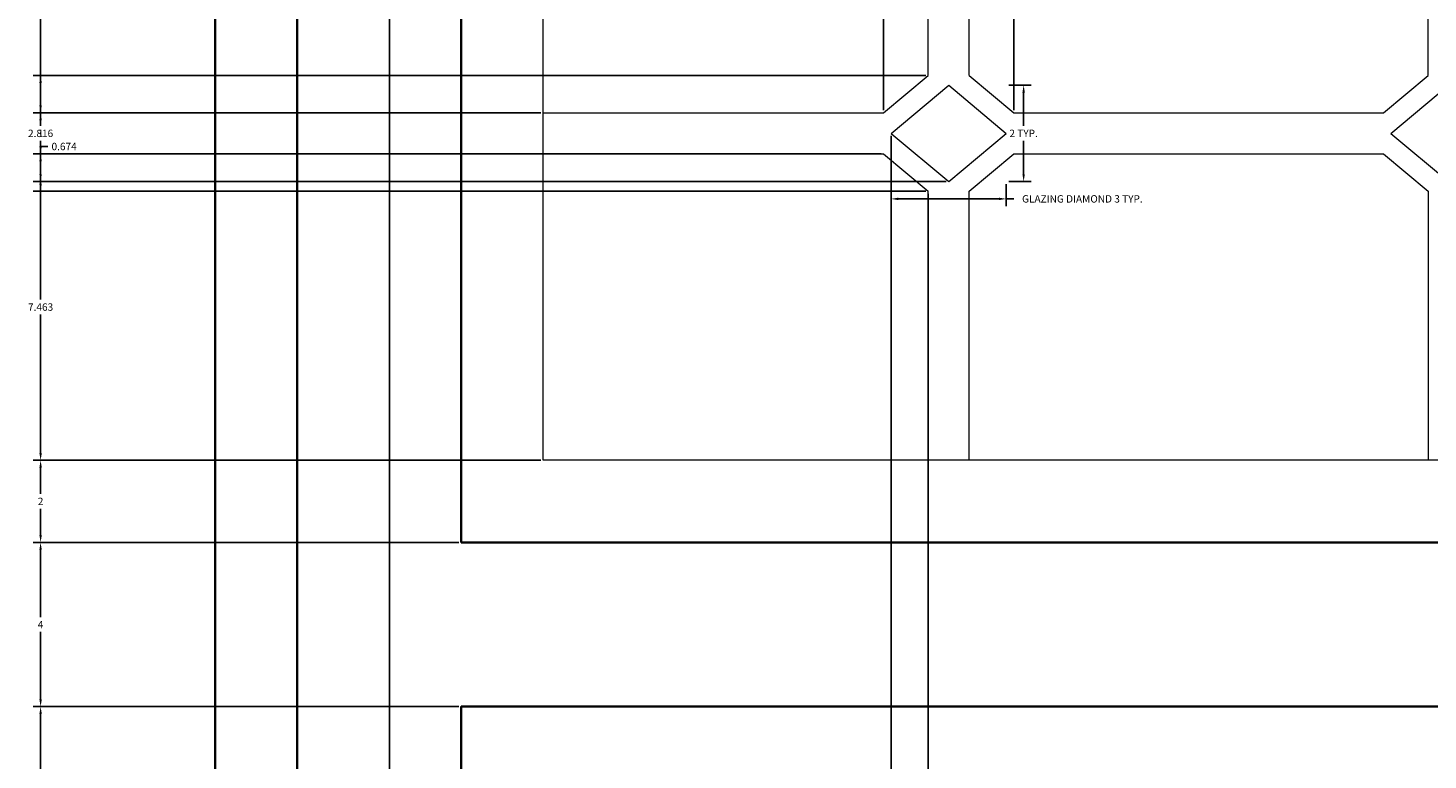
# Model space of a CAD drawing. Units: inches. Extents: x 3137 to 3299, y 1994 to 2089.
# Tile 5 of 14: x 3137 to 3171, y 2052 to 2069. Entities that reach past the tile are written whole.
import ezdxf

# ---------------------------------------------------------------- set-up
doc = ezdxf.new("R2010")
doc.units = ezdxf.units.IN
doc.header["$MEASUREMENT"] = 0
for name, color, linetype, lineweight in [('A-ANNO-DIMS', 2, 'Continuous', 18), ('A-DOOR', 4, 'Continuous', 35), ('A-GLAZ', 3, 'Continuous', 18)]:
    doc.layers.add(name, color=color, linetype=linetype, lineweight=lineweight)
doc.styles.get("Standard").update_dxf_attribs({"font": 'arial.ttf'})
doc.dimstyles.get("Standard").update_dxf_attribs({"dimtxt": 0.18, "dimasz": 0.18, "dimexe": 0.18, "dimexo": 0.0625, "dimgap": 0.09, "dimtad": 0, "dimtih": 1, "dimtoh": 1, "dimdec": 4, "dimzin": 0, "dimdsep": 46, "dimtxsty": 'Standard', "dimcen": 0.09, "dimadec": 0, "dimazin": 0, "dimtfac": 1, "dimtdec": 4, "dimtofl": 0, "dimtmove": 0, "dimatfit": 3, "dimfxl": 1, "dimtolj": 1, "dimtzin": 0, "dimarcsym": 0})

# ---------------------------------------------------------------- blocks, each defined once
blk = doc.blocks.new('GLAZ-DIAMOND-MOTIF')
for points in [[(0, 1.174), (1.407, 2.349)], [(1.407, 2.349), (2.809, 1.174)], [(0, 1.174), (1.407, 0)], [(1.407, 0), (2.809, 1.174)]]:
    blk.add_lwpolyline(points)
blk = doc.blocks.new('*D11')
at = {"layer": 'A-ANNO-DIMS', "color": 0, "lineweight": -2, "transparency": 16777216}
for p, q in [((3157.951, 2065.674), (3157.951, 2065.135)), ((3160.76, 2065.674), (3160.76, 2065.135)), ((3158.131, 2065.315), (3160.58, 2065.315)), ((3160.76, 2065.315), (3160.94, 2065.315))]:
    blk.add_line(p, q, dxfattribs=at)
at = {"layer": 'A-ANNO-DIMS', "color": 0, "transparency": 16777216}
for points in [[(3158.131, 2065.345), (3158.131, 2065.285), (3157.951, 2065.315)], [(3160.58, 2065.345), (3160.58, 2065.285), (3160.76, 2065.315)]]:
    blk.add_solid(points, dxfattribs=at)
at = {"layer": 'Defpoints', "color": 0, "transparency": 16777216}
for p in [(3157.951, 2065.737), (3160.76, 2065.737), (3160.76, 2065.315)]:
    blk.add_point(p, dxfattribs=at)
at = {"layer": 'A-ANNO-DIMS', "color": 0, "transparency": 16777216, "insert": (3162.613, 2065.315), "char_height": 0.18, "attachment_point": 5}
blk.add_mtext('\\A1;GLAZING DIAMOND 3 TYP.', dxfattribs=at)
blk = doc.blocks.new('*D12')
at = {"layer": 'A-ANNO-DIMS', "color": 0, "lineweight": -2, "transparency": 16777216}
for p, q in [((3160.823, 2068.086), (3161.362, 2068.086)), ((3161.182, 2067.906), (3161.182, 2067.092)), ((3161.182, 2065.917), (3161.182, 2066.731)), ((3160.823, 2065.737), (3161.362, 2065.737))]:
    blk.add_line(p, q, dxfattribs=at)
at = {"layer": 'A-ANNO-DIMS', "color": 0, "transparency": 16777216}
for points in [[(3161.152, 2067.906), (3161.212, 2067.906), (3161.182, 2068.086)], [(3161.152, 2065.917), (3161.212, 2065.917), (3161.182, 2065.737)]]:
    blk.add_solid(points, dxfattribs=at)
at = {"layer": 'Defpoints', "color": 0, "transparency": 16777216}
for p in [(3160.76, 2068.086), (3161.182, 2068.086), (3160.76, 2065.737)]:
    blk.add_point(p, dxfattribs=at)
at = {"layer": 'A-ANNO-DIMS', "color": 0, "transparency": 16777216, "insert": (3161.182, 2066.911), "char_height": 0.18, "attachment_point": 5}
blk.add_mtext('\\A1;2 TYP.', dxfattribs=at)
blk = doc.blocks.new('*D42')
at = {"layer": 'A-ANNO-DIMS', "color": 0, "lineweight": -2, "transparency": 16777216}
for p, q in [((3147.415, 2052.948), (3137.048, 2052.948)), ((3137.228, 2052.768), (3137.228, 2042.725)), ((3137.228, 2032.318), (3137.228, 2042.361)), ((3147.415, 2032.138), (3137.048, 2032.138))]:
    blk.add_line(p, q, dxfattribs=at)
at = {"layer": 'A-ANNO-DIMS', "color": 0, "transparency": 16777216}
for points in [[(3137.198, 2052.768), (3137.258, 2052.768), (3137.228, 2052.948)], [(3137.198, 2032.318), (3137.258, 2032.318), (3137.228, 2032.138)]]:
    blk.add_solid(points, dxfattribs=at)
at = {"layer": 'Defpoints', "color": 0, "transparency": 16777216}
for p in [(3137.228, 2052.948), (3147.478, 2052.948), (3147.478, 2032.138)]:
    blk.add_point(p, dxfattribs=at)
at = {"layer": 'A-ANNO-DIMS', "color": 0, "transparency": 16777216, "insert": (3137.228, 2042.543), "char_height": 0.18, "attachment_point": 5}
blk.add_mtext('\\A1;20.81', dxfattribs=at)
blk = doc.blocks.new('*D43')
at = {"layer": 'A-ANNO-DIMS', "color": 0, "lineweight": -2, "transparency": 16777216}
for p, q in [((3147.415181, 2056.948298), (3137.047681, 2056.948298)), ((3137.227681, 2056.768298), (3137.227681, 2055.128298)), ((3137.227681, 2053.128298), (3137.227681, 2054.768298)), ((3147.415181, 2052.948298), (3137.047681, 2052.948298))]:
    blk.add_line(p, q, dxfattribs=at)
at = {"layer": 'A-ANNO-DIMS', "color": 0, "transparency": 16777216}
for points in [[(3137.197681, 2056.768298), (3137.257681, 2056.768298), (3137.227681, 2056.948298)], [(3137.197681, 2053.128298), (3137.257681, 2053.128298), (3137.227681, 2052.948298)]]:
    blk.add_solid(points, dxfattribs=at)
at = {"layer": 'Defpoints', "color": 0, "transparency": 16777216}
for p in [(3137.227681, 2056.948298), (3147.477681, 2056.948298), (3147.477681, 2052.948298)]:
    blk.add_point(p, dxfattribs=at)
at = {"layer": 'A-ANNO-DIMS', "color": 0, "transparency": 16777216, "insert": (3137.227681, 2054.948298), "char_height": 0.18, "attachment_point": 5}
blk.add_mtext('\\A1;4', dxfattribs=at)
blk = doc.blocks.new('*D44')
at = {"layer": 'A-ANNO-DIMS', "color": 0, "lineweight": -2, "transparency": 16777216}
for p, q in [((3149.415, 2058.948), (3137.048, 2058.948)), ((3137.228, 2058.768), (3137.228, 2058.129)), ((3137.228, 2057.128), (3137.228, 2057.768)), ((3147.415, 2056.948), (3137.048, 2056.948))]:
    blk.add_line(p, q, dxfattribs=at)
at = {"layer": 'A-ANNO-DIMS', "color": 0, "transparency": 16777216}
for points in [[(3137.198, 2058.768), (3137.258, 2058.768), (3137.228, 2058.948)], [(3137.198, 2057.128), (3137.258, 2057.128), (3137.228, 2056.948)]]:
    blk.add_solid(points, dxfattribs=at)
at = {"layer": 'Defpoints', "color": 0, "transparency": 16777216}
for p in [(3137.228, 2058.948), (3149.478, 2058.948), (3147.478, 2056.948)]:
    blk.add_point(p, dxfattribs=at)
at = {"layer": 'A-ANNO-DIMS', "color": 0, "transparency": 16777216, "insert": (3137.228, 2057.948), "char_height": 0.18, "attachment_point": 5}
blk.add_mtext('\\A1;2', dxfattribs=at)
blk = doc.blocks.new('*D45')
at = {"layer": 'A-ANNO-DIMS', "color": 0, "lineweight": -2, "transparency": 16777216}
for p, q in [((3149.415, 2066.411), (3137.048, 2066.411)), ((3137.228, 2066.231), (3137.228, 2062.862)), ((3137.228, 2059.128), (3137.228, 2062.498)), ((3149.415, 2058.948), (3137.048, 2058.948))]:
    blk.add_line(p, q, dxfattribs=at)
at = {"layer": 'A-ANNO-DIMS', "color": 0, "transparency": 16777216}
for points in [[(3137.198, 2066.231), (3137.258, 2066.231), (3137.228, 2066.411)], [(3137.198, 2059.128), (3137.258, 2059.128), (3137.228, 2058.948)]]:
    blk.add_solid(points, dxfattribs=at)
at = {"layer": 'Defpoints', "color": 0, "transparency": 16777216}
for p in [(3137.228, 2066.411), (3149.478, 2066.411), (3149.478, 2058.948)]:
    blk.add_point(p, dxfattribs=at)
at = {"layer": 'A-ANNO-DIMS', "color": 0, "transparency": 16777216, "insert": (3137.228, 2062.68), "char_height": 0.18, "attachment_point": 5}
blk.add_mtext('\\A1;7.463', dxfattribs=at)
blk = doc.blocks.new('*D46')
at = {"layer": 'A-ANNO-DIMS', "color": 0, "lineweight": -2, "transparency": 16777216}
for p, q in [((3149.415, 2067.411), (3137.048, 2067.411)), ((3137.228, 2067.231), (3137.228, 2067.092)), ((3137.228, 2066.591), (3137.228, 2066.731)), ((3149.415, 2066.411), (3137.048, 2066.411))]:
    blk.add_line(p, q, dxfattribs=at)
at = {"layer": 'A-ANNO-DIMS', "color": 0, "transparency": 16777216}
for points in [[(3137.198, 2067.231), (3137.258, 2067.231), (3137.228, 2067.411)], [(3137.198, 2066.591), (3137.258, 2066.591), (3137.228, 2066.411)]]:
    blk.add_solid(points, dxfattribs=at)
at = {"layer": 'Defpoints', "color": 0, "transparency": 16777216}
for p in [(3137.228, 2067.411), (3149.478, 2067.411), (3149.478, 2066.411)]:
    blk.add_point(p, dxfattribs=at)
at = {"layer": 'A-ANNO-DIMS', "color": 0, "transparency": 16777216, "insert": (3137.228, 2066.911), "char_height": 0.18, "attachment_point": 5}
blk.add_mtext('\\A1;1', dxfattribs=at)
blk = doc.blocks.new('*D47')
at = {"layer": 'A-ANNO-DIMS', "color": 0, "lineweight": -2, "transparency": 16777216}
for p, q in [((3149.415, 2074.874), (3137.048, 2074.874)), ((3137.228, 2074.694), (3137.228, 2071.325)), ((3137.228, 2067.591), (3137.228, 2070.961)), ((3149.415, 2067.411), (3137.048, 2067.411))]:
    blk.add_line(p, q, dxfattribs=at)
at = {"layer": 'A-ANNO-DIMS', "color": 0, "transparency": 16777216}
for points in [[(3137.198, 2074.694), (3137.258, 2074.694), (3137.228, 2074.874)], [(3137.198, 2067.591), (3137.258, 2067.591), (3137.228, 2067.411)]]:
    blk.add_solid(points, dxfattribs=at)
at = {"layer": 'Defpoints', "color": 0, "transparency": 16777216}
for p in [(3137.228, 2074.874), (3149.478, 2074.874), (3149.478, 2067.411)]:
    blk.add_point(p, dxfattribs=at)
at = {"layer": 'A-ANNO-DIMS', "color": 0, "transparency": 16777216, "insert": (3137.228, 2071.143), "char_height": 0.18, "attachment_point": 5}
blk.add_mtext('\\A1;7.463', dxfattribs=at)
blk = doc.blocks.new('*D55')
at = {"layer": 'A-ANNO-DIMS', "color": 0, "lineweight": -2, "transparency": 16777216}
for p, q in [((3141.54, 2082.874), (3145.908, 2082.874)), ((3145.728, 2082.694), (3145.728, 2041.056)), ((3145.728, 1999.054), (3145.728, 2040.692)), ((3141.54, 1998.874), (3145.908, 1998.874))]:
    blk.add_line(p, q, dxfattribs=at)
at = {"layer": 'A-ANNO-DIMS', "color": 0, "transparency": 16777216}
for points in [[(3145.698, 2082.694), (3145.758, 2082.694), (3145.728, 2082.874)], [(3145.698, 1999.054), (3145.758, 1999.054), (3145.728, 1998.874)]]:
    blk.add_solid(points, dxfattribs=at)
at = {"layer": 'Defpoints', "color": 0, "transparency": 16777216}
for p in [(3141.478, 2082.874), (3141.478, 1998.874), (3145.728, 1998.874)]:
    blk.add_point(p, dxfattribs=at)
at = {"layer": 'A-ANNO-DIMS', "color": 0, "transparency": 16777216, "insert": (3145.728, 2040.874), "char_height": 0.18, "attachment_point": 5}
blk.add_mtext('\\A1;84', dxfattribs=at)
blk = doc.blocks.new('*D79')
at = {"layer": 'A-ANNO-DIMS', "color": 0, "lineweight": -2, "transparency": 16777216}
for p, q in [((3157.769, 2067.474), (3157.769, 2087.304)), ((3157.949, 2087.124), (3158.962, 2087.124)), ((3160.762, 2087.124), (3159.749, 2087.124)), ((3160.942, 2067.474), (3160.942, 2087.304))]:
    blk.add_line(p, q, dxfattribs=at)
at = {"layer": 'A-ANNO-DIMS', "color": 0, "transparency": 16777216}
for points in [[(3157.949, 2087.154), (3157.949, 2087.094), (3157.769, 2087.124)], [(3160.762, 2087.154), (3160.762, 2087.094), (3160.942, 2087.124)]]:
    blk.add_solid(points, dxfattribs=at)
at = {"layer": 'Defpoints', "color": 0, "transparency": 16777216}
for p in [(3160.942, 2087.124), (3157.769, 2067.411), (3160.942, 2067.411)]:
    blk.add_point(p, dxfattribs=at)
at = {"layer": 'A-ANNO-DIMS', "color": 0, "transparency": 16777216, "insert": (3159.356, 2087.124), "char_height": 0.18, "attachment_point": 5}
blk.add_mtext('\\A1;3.173', dxfattribs=at)
blk = doc.blocks.new('*D80')
at = {"layer": 'A-ANNO-DIMS', "color": 0, "lineweight": -2, "transparency": 16777216}
for p, q in [((3158.795, 2068.319), (3137.048, 2068.319)), ((3137.228, 2068.139), (3137.228, 2067.093)), ((3137.228, 2065.683), (3137.228, 2066.729)), ((3158.795, 2065.503), (3137.048, 2065.503))]:
    blk.add_line(p, q, dxfattribs=at)
at = {"layer": 'A-ANNO-DIMS', "color": 0, "transparency": 16777216}
for points in [[(3137.198, 2068.139), (3137.258, 2068.139), (3137.228, 2068.319)], [(3137.198, 2065.683), (3137.258, 2065.683), (3137.228, 2065.503)]]:
    blk.add_solid(points, dxfattribs=at)
at = {"layer": 'Defpoints', "color": 0, "transparency": 16777216}
for p in [(3137.228, 2068.319), (3158.858, 2068.319), (3158.858, 2065.503)]:
    blk.add_point(p, dxfattribs=at)
at = {"layer": 'A-ANNO-DIMS', "color": 0, "transparency": 16777216, "insert": (3137.228, 2066.911), "char_height": 0.18, "attachment_point": 5}
blk.add_mtext('\\A1;2.816', dxfattribs=at)
blk = doc.blocks.new('*D81')
at = {"layer": 'A-ANNO-DIMS', "color": 0, "lineweight": -2, "transparency": 16777216}
for p, q in [((3157.951, 2066.849), (3157.951, 1994.444)), ((3158.858, 2065.44), (3158.858, 1994.444)), ((3157.771, 1994.624), (3157.591, 1994.624)), ((3159.038, 1994.624), (3159.218, 1994.624))]:
    blk.add_line(p, q, dxfattribs=at)
at = {"layer": 'A-ANNO-DIMS', "color": 0, "transparency": 16777216}
for points in [[(3157.771, 1994.654), (3157.771, 1994.594), (3157.951, 1994.624)], [(3159.038, 1994.654), (3159.038, 1994.594), (3158.858, 1994.624)]]:
    blk.add_solid(points, dxfattribs=at)
at = {"layer": 'Defpoints', "color": 0, "transparency": 16777216}
for p in [(3157.951, 2066.911), (3158.858, 2065.503), (3158.858, 1994.624)]:
    blk.add_point(p, dxfattribs=at)
at = {"layer": 'A-ANNO-DIMS', "color": 0, "transparency": 16777216, "insert": (3158.404, 1994.624), "char_height": 0.18, "attachment_point": 5}
blk.add_mtext('\\A1;0.907', dxfattribs=at)
blk = doc.blocks.new('*D82')
at = {"layer": 'A-ANNO-DIMS', "color": 0, "lineweight": -2, "transparency": 16777216}
for p, q in [((3157.707, 2066.411), (3137.048, 2066.411)), ((3137.228, 2066.411), (3137.228, 2066.591)), ((3137.228, 2066.591), (3137.408, 2066.591)), ((3137.228, 2065.917), (3137.228, 2066.231)), ((3159.296, 2065.737), (3137.048, 2065.737))]:
    blk.add_line(p, q, dxfattribs=at)
at = {"layer": 'A-ANNO-DIMS', "color": 0, "transparency": 16777216}
for points in [[(3137.198, 2066.231), (3137.258, 2066.231), (3137.228, 2066.411)], [(3137.198, 2065.917), (3137.258, 2065.917), (3137.228, 2065.737)]]:
    blk.add_solid(points, dxfattribs=at)
at = {"layer": 'Defpoints', "color": 0, "transparency": 16777216}
for p in [(3137.228, 2066.411), (3157.769, 2066.411), (3159.358, 2065.737)]:
    blk.add_point(p, dxfattribs=at)
at = {"layer": 'A-ANNO-DIMS', "color": 0, "transparency": 16777216, "insert": (3137.801, 2066.591), "char_height": 0.18, "attachment_point": 5}
blk.add_mtext('\\A1;0.674', dxfattribs=at)

msp = doc.modelspace()

# ---------------------------------------------------------------- linework, layer by layer
at = {"layer": 'A-DOOR'}
for points in [[(3141.4777, 2082.874), (3189.4777, 2082.874), (3189.4777, 1998.874), (3141.4777, 1998.874)], [(3147.4777, 2056.9483), (3147.4777, 2076.874), (3183.4777, 2076.874), (3183.4777, 2056.9483)], [(3147.4777, 2032.1375), (3147.4777, 2052.9483), (3183.4777, 2052.9483), (3183.4777, 2032.1375)]]:
    msp.add_lwpolyline(points, close=True, dxfattribs=at)
msp.add_lwpolyline([(3187.4777, 2007.6773), (3187.4777, 2000.874), (3143.4777, 2000.874), (3143.4777, 2080.874), (3187.4777, 2080.874), (3187.4777, 2076.298)], dxfattribs=at)
at = {"layer": 'A-GLAZ'}
for p, q in [((3158.8577, 2068.3193), (3158.8577, 2074.874)), ((3159.8577, 2068.3193), (3159.8577, 2074.874)), ((3171.0351, 2068.3193), (3171.0351, 2074.874)), ((3149.4777, 2067.4111), (3157.7694, 2067.4111)), ((3160.9422, 2067.4111), (3169.9468, 2067.4111)), ((3149.4777, 2066.4111), (3157.7694, 2066.4111)), ((3160.9422, 2066.4111), (3169.9468, 2066.4111)), ((3158.8577, 2058.9483), (3158.8577, 2065.5029)), ((3159.8577, 2058.9483), (3159.8577, 2065.5029)), ((3171.0351, 2065.5029), (3171.0351, 2058.9483))]:
    msp.add_line(p, q, dxfattribs=at)
msp.add_lwpolyline([(3149.4777, 2058.9483), (3149.4777, 2074.874), (3181.4777, 2074.874), (3181.4777, 2058.9483)], close=True, dxfattribs=at)
for points in [[(3157.7694, 2067.4111), (3158.8577, 2068.3193)], [(3159.8577, 2068.3193), (3160.9422, 2067.4111)], [(3169.9468, 2067.4111), (3171.0351, 2068.3193)], [(3157.7694, 2066.4111), (3158.8577, 2065.5029)], [(3159.8577, 2065.5029), (3160.9422, 2066.4111)], [(3169.9468, 2066.4111), (3171.0351, 2065.5029)]]:
    msp.add_lwpolyline(points, dxfattribs=at)

# ---------------------------------------------------------------- block references
for p in [(3157.951, 2065.737), (3170.1284, 2065.737)]:
    msp.add_blockref('GLAZ-DIAMOND-MOTIF', p, dxfattribs=at)

# ---------------------------------------------------------------- dimensions: what is measured, and where the dimension line sits
at = {"layer": 'A-ANNO-DIMS'}
for base, p1, p2, picture, middle in [((3160.9422, 2087.124), (3157.7694, 2067.4111), (3160.9422, 2067.4111), '*D79', (3159.3558, 2087.124)), ((3158.8577, 1994.624), (3157.9507, 2066.9111), (3158.8577, 2065.5029), '*D81', (3158.4042, 1994.624))]:
    dim = msp.add_linear_dim(base=base, p1=p1, p2=p2, dimstyle='Standard', override={"dimdec": 3, "dimlfac": 1, "dimrnd": 0, "dimzin": 0, "dimdsep": 46, "dimlunit": 2}, dxfattribs=at)
    dim.commit()
    dim.dimension.update_dxf_attribs({"geometry": picture, "text_midpoint": middle})
for base, p1, p2, angle, override, picture, middle in [((3145.7277, 1998.874), (3141.4777, 2082.874), (3141.4777, 1998.874), 270, {"dimdec": 0, "dimlfac": 1, "dimrnd": 0, "dimzin": 0, "dimdsep": 46, "dimlunit": 2}, '*D55', (3145.7277, 2040.874)), ((3137.2277, 2074.874), (3149.4777, 2067.4111), (3149.4777, 2074.874), 90, {"dimdec": 3, "dimlfac": 1, "dimrnd": 0, "dimzin": 0, "dimdsep": 46, "dimlunit": 2}, '*D47', (3137.2277, 2071.1426)), ((3137.2277, 2068.3193), (3158.8577, 2065.5029), (3158.8577, 2068.3193), 90, {"dimdec": 3, "dimlfac": 1, "dimrnd": 0, "dimzin": 0, "dimdsep": 46, "dimlunit": 2}, '*D80', (3137.2277, 2066.9111)), ((3137.2277, 2067.4111), (3149.4777, 2066.4111), (3149.4777, 2067.4111), 90, {"dimdec": 0, "dimlfac": 1, "dimrnd": 0, "dimzin": 0, "dimdsep": 46, "dimlunit": 2}, '*D46', (3137.2277, 2066.9111)), ((3137.22768, 2066.41113), (3159.358, 2065.73665), (3157.76944, 2066.41113), 90, {"dimdec": 3, "dimlfac": 1, "dimrnd": 0, "dimzin": 0, "dimdsep": 46, "dimlunit": 2}, '*D82', (3137.80102, 2066.59113)), ((3137.2277, 2066.4111), (3149.4777, 2058.9483), (3149.4777, 2066.4111), 90, {"dimdec": 3, "dimlfac": 1, "dimrnd": 0, "dimzin": 0, "dimdsep": 46, "dimlunit": 2}, '*D45', (3137.2277, 2062.6797)), ((3137.2277, 2058.9483), (3147.4777, 2056.9483), (3149.4777, 2058.9483), 90, {"dimdec": 0, "dimlfac": 1, "dimrnd": 0, "dimzin": 0, "dimdsep": 46, "dimlunit": 2}, '*D44', (3137.2277, 2057.9483)), ((3137.2277, 2056.9483), (3147.4777, 2052.9483), (3147.4777, 2056.9483), 90, {"dimdec": 0, "dimlfac": 1, "dimrnd": 0, "dimzin": 0, "dimdsep": 46, "dimlunit": 2}, '*D43', (3137.2277, 2054.9483)), ((3137.2277, 2052.9483), (3147.4777, 2032.1375), (3147.4777, 2052.9483), 90, {"dimdec": 2, "dimlfac": 1, "dimrnd": 0, "dimzin": 0, "dimdsep": 46, "dimlunit": 2}, '*D42', (3137.2277, 2042.5429))]:
    dim = msp.add_linear_dim(base=base, p1=p1, p2=p2, angle=angle, dimstyle='Standard', override=override, dxfattribs=at)
    dim.commit()
    dim.dimension.update_dxf_attribs({"geometry": picture, "text_midpoint": middle})
dim = msp.add_linear_dim(base=(3161.182, 2068.0856), p1=(3160.7605, 2065.7366), p2=(3160.7605, 2068.0856), angle=90, text='<> TYP.', dimstyle='Standard', override={"dimdec": 0, "dimrnd": 0, "dimzin": 0, "dimlunit": 2}, dxfattribs=at)
dim.commit()
dim.dimension.update_dxf_attribs({"geometry": '*D12', "text_midpoint": (3161.182, 2066.9111)})
dim = msp.add_linear_dim(base=(3160.7605, 2065.3152), p1=(3157.9507, 2065.7366), p2=(3160.7605, 2065.7366), text='GLAZING DIAMOND <> TYP.', dimstyle='Standard', override={"dimdec": 0, "dimrnd": 0, "dimzin": 0, "dimlunit": 2}, dxfattribs=at)
dim.commit()
dim.dimension.update_dxf_attribs({"geometry": '*D11', "text_midpoint": (3162.6127, 2065.3152)})

doc.saveas('drawing.dxf')
